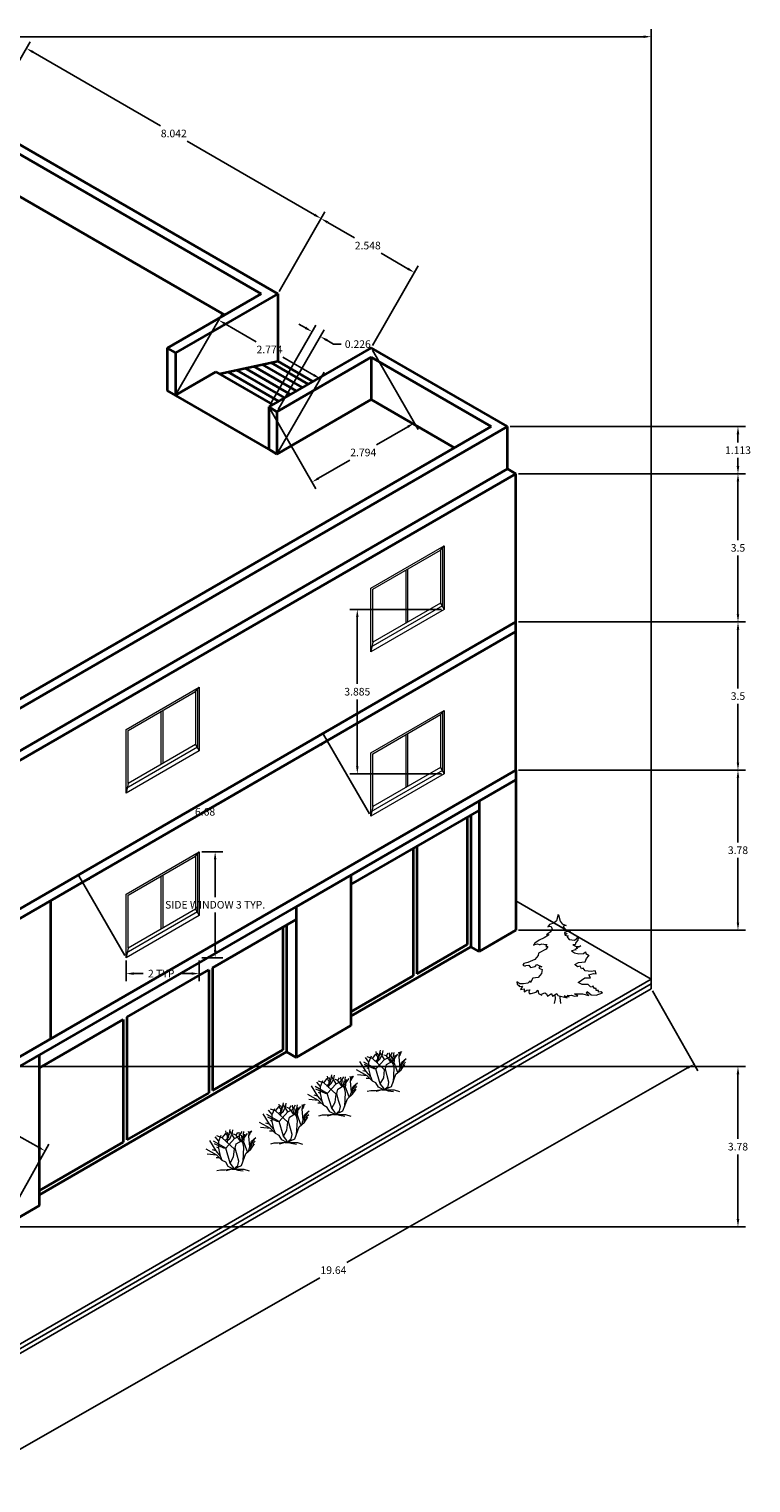
# Model space of a CAD drawing. Units: metres. Extents: x 5057 to 10150, y 1364 to 2760.
# Tile 2 of 2: x 5082 to 5099, y 1364 to 1399. Entities that reach past the tile are written whole.
import ezdxf

# ---------------------------------------------------------------- set-up
doc = ezdxf.new("R2010")
doc.units = ezdxf.units.M
for name, color, linetype, lineweight in [('A-ANNO-DIMS', 2, 'Continuous', 18), ('A-ELEV', 7, 'Continuous', 35), ('A-GLAZ', 4, 'Continuous', 18), ('C-SITE', 3, 'Continuous', 25), ('L-PLNT', 3, 'Continuous', 13)]:
    doc.layers.add(name, color=color, linetype=linetype, lineweight=lineweight)
doc.styles.get("Standard").update_dxf_attribs({"font": 'arial.ttf'})
doc.dimstyles.get("Standard").update_dxf_attribs({"dimtxt": 0.18, "dimasz": 0.18, "dimexe": 0.18, "dimexo": 0.0625, "dimgap": 0.09, "dimtad": 0, "dimtih": 1, "dimtoh": 1, "dimdec": 4, "dimzin": 0, "dimdsep": 46, "dimtxsty": 'Standard', "dimcen": 0.09, "dimadec": 0, "dimazin": 0, "dimtfac": 1, "dimtdec": 4, "dimtofl": 0, "dimtmove": 0, "dimatfit": 3, "dimfxl": 1, "dimtolj": 1, "dimtzin": 0, "dimarcsym": 0})

# ---------------------------------------------------------------- blocks, each defined once
blk = doc.blocks.new('*U4')
for p, q in [((-18.24, 11.04), (-21.755, 16.655)), ((-12.96, 12.48), (-19.68, 16.32)), ((-16.8, 16.32), (-18.72, 18.72)), ((-14.88, 18.24), (-17.76, 19.2)), ((-16.8, 16.32), (-15.36, 19.68)), ((-16.8, 12.48), (-16.8, 16.32)), ((-14.88, 18.24), (-12.96, 20.64)), ((-8.16, 12), (-14.88, 18.24)), ((-13.325, 16.724), (-11.433, 18.289)), ((-12.96, 12.48), (-8.16, 17.76)), ((-12.471, 19.775), (-12.898, 22.044)), ((-11.677, 19.071), (-12.471, 19.775)), ((-11.28, 19.619), (-12.104, 21.184)), ((-12.043, 15.628), (-11.921, 18.836)), ((-11.982, 16.802), (-10.579, 18.054)), ((-11.921, 18.836), (-10.64, 20.401)), ((-11.433, 18.289), (-10.457, 22.749)), ((-10.579, 18.054), (-9.846, 19.697)), ((-8.16, 17.76), (-10.56, 21.6)), ((-9.48, 19.775), (-8.992, 22.592)), ((-7.2, 19.68), (-8.64, 20.16)), ((-8.16, 17.76), (-5.28, 19.2)), ((-7.2, 19.68), (-6.24, 21.12)), ((-4.8, 16.32), (-7.2, 19.68)), ((-7.2, 14.88), (-3.84, 16.8)), ((-5.086, 17.741), (-5.513, 21.34)), ((-5.28, 19.2), (-3.84, 21.6)), ((-3.377, 15.315), (-5.086, 17.819)), ((-2.88, 12.96), (-4.32, 19.68)), ((-3.84, 16.8), (-0.96, 20.64)), ((-3.377, 18.602), (-2.888, 21.575)), ((-2.766, 16.802), (-3.377, 18.602)), ((-2.88, 15.84), (-2.4, 20.16)), ((-0.508, 21.888), (-0.081, 20.558)), ((-0.203, 19.149), (0.102, 21.34)), ((0.346, 13.203), (-0.203, 19.149)), ((-0.142, 19.384), (0.59, 20.401)), ((-0.02, 20.01), (0.896, 21.105)), ((0.041, 20.714), (1.384, 22.044)), ((0.102, 21.34), (0.835, 21.888)), ((0.346, 13.203), (1.323, 16.254)), ((1.323, 16.254), (3.642, 18.289)), ((1.44, 15.36), (2.88, 17.28)), ((2.4, 15.36), (3.36, 16.32)), ((-17.76, 8.64), (-23.663, 11.961)), ((-17.76, 8.64), (-23.128, 9.222)), ((-18.24, 11.04), (-20.16, 11.52)), ((-13.92, 12.48), (-19.2, 14.88)), ((-15.84, 8.16), (-18.24, 11.04)), ((-16.8, 12.48), (-17.76, 12.96)), ((-14.88, 5.76), (-17.76, 8.64)), ((-15.84, 8.16), (-16.8, 12.48)), ((-14.88, 5.76), (-15.84, 8.16)), ((-12.96, 12.48), (-13.92, 12.48)), ((-10.56, 4.32), (-12.96, 12.48)), ((-8.64, 7.68), (-8.16, 12)), ((-7.68, 12.48), (-7.2, 14.88)), ((-6.72, 8.64), (-7.68, 12.48)), ((-5.76, 5.28), (-6.72, 8.64)), ((-4.32, 2.88), (-1.92, 9.6)), ((-3.36, 5.28), (-2.88, 12.96)), ((-0.96, 10.56), (-2.88, 15.84)), ((-1.92, 9.6), (0.96, 12)), ((-0.48, 10.8), (0.346, 13.203)), ((0.96, 12), (1.44, 15.36)), ((0.96, 12), (2.88, 14.88)), ((1.92, 13.44), (2.4, 15.36)), ((-16.32, 7.2), (-18.24, 7.2)), ((-15.84, 0.48), (-17.76, 0)), ((-13.44, 0.48), (-15.84, 0.48)), ((-12.96, 4.8), (-14.88, 5.76)), ((-9.6, 0.96), (-13.44, 0.48)), ((-11.52, 2.4), (-12.96, 4.8)), ((-9.6, 0.96), (-12.96, 0)), ((-8.64, 0.96), (-11.52, 2.4)), ((-10.56, 4.32), (-8.64, 7.68)), ((-8.64, 1.92), (-10.56, 4.32)), ((-9.6, 0.96), (-7.68, 0.96)), ((-8.64, 0.96), (-4.32, 2.88)), ((-8.64, 0.96), (-6.24, 2.88)), ((-8.64, 0.96), (-8.64, 1.92)), ((-8.64, 0.96), (-2.88, 0.96)), ((-7.68, 0.96), (-6.24, 0.48)), ((-6.24, 2.88), (-5.76, 5.28)), ((-6.24, 0.48), (-3.36, 0)), ((-2.88, 0.96), (0, 0))]:
    blk.add_line(p, q)
blk = doc.blocks.new('*U5')
for p, q in [((-9.75, 0), (-8.263, 7.598)), ((-8.263, 7.598), (-8.747, 14.105)), ((-0.771, 9.56), (-0.69, 11.833)), ((0, 0), (-0.771, 9.56))]:
    blk.add_line(p, q)
for points in [[(-3.9, 142.35), (-6.596, 132.037), (-10.801, 128.443), (-17.81, 126.047), (-20.614, 122.452), (-17.81, 123.65), (-15.007, 123.051), (-13.605, 118.858), (-16.876, 114.065), (-21.549, 111.07), (-22.951, 109.872), (-19.212, 110.471), (-19.68, 109.273), (-26.222, 105.079), (-34.633, 101.485), (-41.175, 96.693), (-43.511, 93.098), (-41.175, 94.296), (-36.969, 95.494), (-34.633, 94.296), (-32.764, 94.296), (-29.493, 95.494)], [(-3.759, 141.97), (-1.074, 131.643), (2.437, 127.141), (8.84, 124.493), (6.568, 124.493), (4.09, 123.169), (4.296, 121.846), (7.807, 117.874), (16.069, 116.02), (10.492, 115.226), (5.535, 113.372), (6.981, 112.843), (5.948, 110.989), (10.286, 112.048), (6.775, 109.401), (11.732, 108.077), (9.873, 107.282), (13.797, 102.516), (21.852, 101.192), (25.983, 103.84), (28.048, 106.488), (27.842, 105.164), (27.429, 101.457), (24.124, 97.75), (23.091, 93.513), (19.58, 93.513), (23.505, 91.66), (28.255, 90.866), (31.973, 91.925), (29.081, 89.806), (24.537, 88.747), (26.809, 88.218), (22.472, 86.099), (24.95, 85.57), (17.308, 84.246), (21.852, 80.804), (29.081, 79.215), (36.723, 80.009), (39.821, 82.392), (40.028, 80.009), (45.398, 76.567)], [(-29.25, 95.55), (-25.287, 94.296), (-22.016, 94.296), (-23.885, 91.301), (-20.614, 91.301), (-23.418, 87.108), (-35.567, 80.518), (-36.035, 76.924), (-41.175, 70.334), (-52.389, 65.542), (-58.931, 63.744), (-60.8, 61.348), (-57.062, 59.551), (-56.128, 60.749), (-50.987, 61.348), (-48.184, 57.754), (-40.707, 58.952), (-38.371, 62.546), (-30.427, 58.353), (-33.698, 58.353), (-35.1, 56.556), (-29.493, 54.159), (-30.894, 48.169), (-36.035, 41.579), (-44.446, 40.381), (-48.184, 33.791), (-49.118, 36.188), (-52.857, 32.593), (-59.399, 31.395), (-65.473, 31.395), (-70.146, 34.39), (-69.679, 30.796), (-66.875, 28.999), (-65.941, 27.202), (-61.268, 27.801), (-64.539, 22.409), (-58.464, 23.607), (-58.464, 18.815), (-54.258, 21.211), (-49.586, 21.81), (-50.987, 18.815), (-50.52, 15.82), (-47.249, 15.82), (-39.306, 18.216), (-36.502, 21.211), (-35.567, 15.82), (-30.427, 13.423), (-29.493, 15.221), (-25.287, 17.018), (-22.951, 15.221), (-21.081, 11.626), (-14.539, 15.82), (-13.138, 11.626), (-6.128, 15.82), (-4.726, 12.824), (10.226, 9.23), (5.554, 12.225), (13.497, 10.428), (10.226, 12.824), (16.768, 13.423), (22.376, 11.626), (27.516, 12.225), (21.909, 15.221), (34.993, 15.221), (44.806, 12.824), (41.535, 16.419), (42.469, 19.414), (49.011, 14.023), (56.487, 13.423), (66.768, 17.018), (64.431, 18.815), (60.226, 18.216), (60.226, 20.612), (56.955, 20.612), (56.955, 24.206), (54.151, 24.206), (51.348, 28.4), (50.413, 26.004), (47.609, 26.603), (43.871, 30.197), (38.731, 30.197), (34.525, 30.197), (27.983, 33.791), (38.731, 40.98), (47.609, 40.98), (45.273, 45.773), (52.282, 48.169), (56.955, 47.57), (55.086, 52.362), (48.544, 51.164), (39.198, 52.362), (35.927, 56.556), (33.123, 55.357), (31.254, 59.551), (27.049, 58.353), (22.376, 62.546), (28.451, 65.542), (39.198, 66.74), (41.535, 72.131), (45.273, 76.325)]]:
    blk.add_lwpolyline(points)
blk = doc.blocks.new('WIN-SIDE')
for p, q in [((0, 1.5), (1.732, 2.5)), ((1.646, 2.4), (1.732, 2.5)), ((1.692, 2.453), (1.692, 1.083)), ((1.732, 2.5), (1.732, 1)), ((0.049, 1.478), (1.646, 2.4)), ((1.646, 2.4), (1.646, 1.15)), ((0.826, 1.926), (0.826, 0.676)), ((0.869, 1.951), (0.869, 0.701)), ((0, 0), (0, 1.5)), ((0.049, 0.228), (0.049, 1.478)), ((1.692, 1.083), (0, 0.107)), ((1.646, 1.15), (0.049, 0.228)), ((1.646, 1.15), (1.732, 1)), ((1.732, 1), (0, 0)), ((0.049, 0.228), (0, 0))]:
    blk.add_line(p, q)
blk = doc.blocks.new('*D7')
at = {"layer": 'A-ANNO-DIMS', "color": 0, "lineweight": -2, "transparency": 16777216}
for p, q in [((5085.663, 1379.094), (5086.155, 1379.094)), ((5085.975, 1378.914), (5085.975, 1378.027)), ((5085.975, 1376.774), (5085.975, 1377.66)), ((5085.663, 1376.594), (5086.155, 1376.594))]:
    blk.add_line(p, q, dxfattribs=at)
at = {"layer": 'A-ANNO-DIMS', "color": 0, "transparency": 16777216}
for points in [[(5085.945, 1378.914), (5086.005, 1378.914), (5085.975, 1379.094)], [(5085.945, 1376.774), (5086.005, 1376.774), (5085.975, 1376.594)]]:
    blk.add_solid(points, dxfattribs=at)
at = {"layer": 'Defpoints', "color": 0, "transparency": 16777216}
for p in [(5085.6, 1379.094), (5085.975, 1379.094), (5085.6, 1376.594)]:
    blk.add_point(p, dxfattribs=at)
at = {"layer": 'A-ANNO-DIMS', "color": 0, "transparency": 16777216, "insert": (5085.975, 1377.844), "char_height": 0.18, "attachment_point": 5}
blk.add_mtext('\\A1;SIDE WINDOW 3 TYP.', dxfattribs=at)
blk = doc.blocks.new('*D8')
at = {"layer": 'A-ANNO-DIMS', "color": 0, "lineweight": -2, "transparency": 16777216}
for p, q in [((5083.868, 1376.531), (5083.868, 1376.039)), ((5085.6, 1376.531), (5085.6, 1376.039)), ((5084.048, 1376.219), (5084.275, 1376.219)), ((5085.42, 1376.219), (5085.194, 1376.219))]:
    blk.add_line(p, q, dxfattribs=at)
at = {"layer": 'A-ANNO-DIMS', "color": 0, "transparency": 16777216}
for points in [[(5084.048, 1376.249), (5084.048, 1376.189), (5083.868, 1376.219)], [(5085.42, 1376.249), (5085.42, 1376.189), (5085.6, 1376.219)]]:
    blk.add_solid(points, dxfattribs=at)
at = {"layer": 'Defpoints', "color": 0, "transparency": 16777216}
for p in [(5083.868, 1376.594), (5085.6, 1376.594), (5085.6, 1376.219)]:
    blk.add_point(p, dxfattribs=at)
at = {"layer": 'A-ANNO-DIMS', "color": 0, "transparency": 16777216, "insert": (5084.734, 1376.219), "char_height": 0.18, "attachment_point": 5}
blk.add_mtext('\\A1;2 TYP.', dxfattribs=at)
blk = doc.blocks.new('*D9')
at = {"layer": 'A-ANNO-DIMS', "color": 0, "lineweight": -2, "transparency": 16777216}
for p, q in [((5059.194, 1377.756), (5059.194, 1398.523)), ((5059.374, 1398.343), (5077.345, 1398.343)), ((5096.103, 1398.343), (5078.132, 1398.343)), ((5096.283, 1375.925), (5096.283, 1398.523))]:
    blk.add_line(p, q, dxfattribs=at)
at = {"layer": 'A-ANNO-DIMS', "color": 0, "transparency": 16777216}
for points in [[(5059.374, 1398.373), (5059.374, 1398.313), (5059.194, 1398.343)], [(5096.103, 1398.373), (5096.103, 1398.313), (5096.283, 1398.343)]]:
    blk.add_solid(points, dxfattribs=at)
at = {"layer": 'Defpoints', "color": 0, "transparency": 16777216}
for p in [(5096.283, 1398.343), (5059.194, 1377.694), (5096.283, 1375.863)]:
    blk.add_point(p, dxfattribs=at)
at = {"layer": 'A-ANNO-DIMS', "color": 0, "transparency": 16777216, "insert": (5077.738, 1398.343), "char_height": 0.18, "attachment_point": 5}
blk.add_mtext('\\A1;37.09', dxfattribs=at)
blk = doc.blocks.new('*D12')
at = {"layer": 'A-ANNO-DIMS', "color": 0, "lineweight": -2, "transparency": 16777216}
for p, q in [((5096.314, 1375.808), (5097.388, 1373.926)), ((5097.143, 1373.993), (5089.09, 1369.397)), ((5080.399, 1364.437), (5088.452, 1369.033)), ((5079.257, 1366.074), (5080.332, 1364.191))]:
    blk.add_line(p, q, dxfattribs=at)
at = {"layer": 'A-ANNO-DIMS', "color": 0, "transparency": 16777216}
for points in [[(5097.128, 1374.019), (5097.158, 1373.967), (5097.299, 1374.082)], [(5080.384, 1364.463), (5080.414, 1364.411), (5080.243, 1364.348)]]:
    blk.add_solid(points, dxfattribs=at)
at = {"layer": 'Defpoints', "color": 0, "transparency": 16777216}
for p in [(5096.283, 1375.863), (5079.226, 1366.128), (5080.243, 1364.348)]:
    blk.add_point(p, dxfattribs=at)
at = {"layer": 'A-ANNO-DIMS', "color": 0, "transparency": 16777216, "insert": (5088.771, 1369.215), "char_height": 0.18, "attachment_point": 5}
blk.add_mtext('\\A1;19.64', dxfattribs=at)
blk = doc.blocks.new('*D13')
at = {"layer": 'A-ANNO-DIMS', "color": 0, "lineweight": -2, "transparency": 16777216}
for p, q in [((5093.145, 1381.022), (5098.513, 1381.022)), ((5098.333, 1380.842), (5098.333, 1379.314)), ((5098.333, 1377.421), (5098.333, 1378.95)), ((5093.145, 1377.241), (5098.513, 1377.241))]:
    blk.add_line(p, q, dxfattribs=at)
at = {"layer": 'A-ANNO-DIMS', "color": 0, "transparency": 16777216}
for points in [[(5098.303, 1380.842), (5098.363, 1380.842), (5098.333, 1381.022)], [(5098.303, 1377.421), (5098.363, 1377.421), (5098.333, 1377.241)]]:
    blk.add_solid(points, dxfattribs=at)
at = {"layer": 'Defpoints', "color": 0, "transparency": 16777216}
for p in [(5093.083, 1381.022), (5098.333, 1381.022), (5093.083, 1377.241)]:
    blk.add_point(p, dxfattribs=at)
at = {"layer": 'A-ANNO-DIMS', "color": 0, "transparency": 16777216, "insert": (5098.333, 1379.132), "char_height": 0.18, "attachment_point": 5}
blk.add_mtext('\\A1;3.78', dxfattribs=at)
blk = doc.blocks.new('*D14')
at = {"layer": 'A-ANNO-DIMS', "color": 0, "lineweight": -2, "transparency": 16777216}
for p, q in [((5093.145, 1384.522), (5098.513, 1384.522)), ((5098.333, 1384.342), (5098.333, 1382.954)), ((5098.333, 1381.202), (5098.333, 1382.59)), ((5093.145, 1381.022), (5098.513, 1381.022))]:
    blk.add_line(p, q, dxfattribs=at)
at = {"layer": 'A-ANNO-DIMS', "color": 0, "transparency": 16777216}
for points in [[(5098.303, 1384.342), (5098.363, 1384.342), (5098.333, 1384.522)], [(5098.303, 1381.202), (5098.363, 1381.202), (5098.333, 1381.022)]]:
    blk.add_solid(points, dxfattribs=at)
at = {"layer": 'Defpoints', "color": 0, "transparency": 16777216}
for p in [(5093.083, 1384.522), (5098.333, 1384.522), (5093.083, 1381.022)]:
    blk.add_point(p, dxfattribs=at)
at = {"layer": 'A-ANNO-DIMS', "color": 0, "transparency": 16777216, "insert": (5098.333, 1382.772), "char_height": 0.18, "attachment_point": 5}
blk.add_mtext('\\A1;3.5', dxfattribs=at)
blk = doc.blocks.new('*D15')
at = {"layer": 'A-ANNO-DIMS', "color": 0, "lineweight": -2, "transparency": 16777216}
for p, q in [((5093.145, 1388.022), (5098.513, 1388.022)), ((5098.333, 1387.842), (5098.333, 1386.454)), ((5098.333, 1384.702), (5098.333, 1386.09)), ((5093.145, 1384.522), (5098.513, 1384.522))]:
    blk.add_line(p, q, dxfattribs=at)
at = {"layer": 'A-ANNO-DIMS', "color": 0, "transparency": 16777216}
for points in [[(5098.303, 1387.842), (5098.363, 1387.842), (5098.333, 1388.022)], [(5098.303, 1384.702), (5098.363, 1384.702), (5098.333, 1384.522)]]:
    blk.add_solid(points, dxfattribs=at)
at = {"layer": 'Defpoints', "color": 0, "transparency": 16777216}
for p in [(5093.083, 1388.022), (5098.333, 1388.022), (5093.083, 1384.522)]:
    blk.add_point(p, dxfattribs=at)
at = {"layer": 'A-ANNO-DIMS', "color": 0, "transparency": 16777216, "insert": (5098.333, 1386.272), "char_height": 0.18, "attachment_point": 5}
blk.add_mtext('\\A1;3.5', dxfattribs=at)
blk = doc.blocks.new('*D16')
at = {"layer": 'A-ANNO-DIMS', "color": 0, "lineweight": -2, "transparency": 16777216}
for p, q in [((5092.95, 1389.135), (5098.513, 1389.135)), ((5098.333, 1388.955), (5098.333, 1388.761)), ((5098.333, 1388.202), (5098.333, 1388.397)), ((5093.145, 1388.022), (5098.513, 1388.022))]:
    blk.add_line(p, q, dxfattribs=at)
at = {"layer": 'A-ANNO-DIMS', "color": 0, "transparency": 16777216}
for points in [[(5098.303, 1388.955), (5098.363, 1388.955), (5098.333, 1389.135)], [(5098.303, 1388.202), (5098.363, 1388.202), (5098.333, 1388.022)]]:
    blk.add_solid(points, dxfattribs=at)
at = {"layer": 'Defpoints', "color": 0, "transparency": 16777216}
for p in [(5092.887, 1389.135), (5098.333, 1389.135), (5093.083, 1388.022)]:
    blk.add_point(p, dxfattribs=at)
at = {"layer": 'A-ANNO-DIMS', "color": 0, "transparency": 16777216, "insert": (5098.333, 1388.579), "char_height": 0.18, "attachment_point": 5}
blk.add_mtext('\\A1;1.113', dxfattribs=at)
blk = doc.blocks.new('*D17')
at = {"layer": 'A-ANNO-DIMS', "color": 0, "lineweight": -2, "transparency": 16777216}
for p, q in [((5080.521, 1396.347), (5081.604, 1398.224)), ((5081.67, 1397.979), (5084.681, 1396.24)), ((5088.323, 1394.138), (5085.312, 1395.876)), ((5087.485, 1392.327), (5088.569, 1394.204))]:
    blk.add_line(p, q, dxfattribs=at)
at = {"layer": 'A-ANNO-DIMS', "color": 0, "transparency": 16777216}
for points in [[(5081.685, 1398.005), (5081.655, 1397.953), (5081.514, 1398.069)], [(5088.338, 1394.164), (5088.308, 1394.112), (5088.479, 1394.048)]]:
    blk.add_solid(points, dxfattribs=at)
at = {"layer": 'Defpoints', "color": 0, "transparency": 16777216}
for p in [(5080.489, 1396.293), (5088.479, 1394.048), (5087.454, 1392.272)]:
    blk.add_point(p, dxfattribs=at)
at = {"layer": 'A-ANNO-DIMS', "color": 0, "transparency": 16777216, "insert": (5084.997, 1396.058), "char_height": 0.18, "attachment_point": 5}
blk.add_mtext('\\A1;8.042', dxfattribs=at)
blk = doc.blocks.new('*D18')
at = {"layer": 'A-ANNO-DIMS', "color": 0, "lineweight": -2, "transparency": 16777216}
for p, q in [((5087.485, 1392.327), (5088.569, 1394.204)), ((5088.635, 1393.958), (5089.267, 1393.593)), ((5090.529, 1392.864), (5089.897, 1393.229)), ((5089.692, 1391.053), (5090.775, 1392.93))]:
    blk.add_line(p, q, dxfattribs=at)
at = {"layer": 'A-ANNO-DIMS', "color": 0, "transparency": 16777216}
for points in [[(5088.65, 1393.984), (5088.62, 1393.932), (5088.479, 1394.048)], [(5090.544, 1392.89), (5090.514, 1392.838), (5090.685, 1392.774)]]:
    blk.add_solid(points, dxfattribs=at)
at = {"layer": 'Defpoints', "color": 0, "transparency": 16777216}
for p in [(5090.685, 1392.774), (5087.454, 1392.272), (5089.66, 1390.998)]:
    blk.add_point(p, dxfattribs=at)
at = {"layer": 'A-ANNO-DIMS', "color": 0, "transparency": 16777216, "insert": (5089.582, 1393.411), "char_height": 0.18, "attachment_point": 5}
blk.add_mtext('\\A1;2.548', dxfattribs=at)
blk = doc.blocks.new('*D19')
at = {"layer": 'A-ANNO-DIMS', "color": 0, "lineweight": -2, "transparency": 16777216}
for p, q in [((5089.692, 1390.944), (5090.775, 1389.067)), ((5087.272, 1389.547), (5088.356, 1387.67)), ((5090.529, 1389.133), (5089.79, 1388.706)), ((5088.421, 1387.916), (5089.16, 1388.343))]:
    blk.add_line(p, q, dxfattribs=at)
at = {"layer": 'A-ANNO-DIMS', "color": 0, "transparency": 16777216}
for points in [[(5090.514, 1389.159), (5090.544, 1389.107), (5090.685, 1389.223)], [(5088.406, 1387.942), (5088.436, 1387.89), (5088.266, 1387.826)]]:
    blk.add_solid(points, dxfattribs=at)
at = {"layer": 'Defpoints', "color": 0, "transparency": 16777216}
for p in [(5089.66, 1390.998), (5087.241, 1389.601), (5088.266, 1387.826)]:
    blk.add_point(p, dxfattribs=at)
at = {"layer": 'A-ANNO-DIMS', "color": 0, "transparency": 16777216, "insert": (5089.475, 1388.525), "char_height": 0.18, "attachment_point": 5}
blk.add_mtext('\\A1;2.794', dxfattribs=at)
blk = doc.blocks.new('*D20')
at = {"layer": 'A-ANNO-DIMS', "color": 0, "lineweight": -2, "transparency": 16777216}
for p, q in [((5087.272, 1389.655), (5088.356, 1391.533)), ((5088.11, 1391.467), (5087.954, 1391.557)), ((5087.468, 1389.542), (5088.551, 1391.42)), ((5088.617, 1391.174), (5088.773, 1391.084)), ((5088.773, 1391.084), (5088.953, 1391.084))]:
    blk.add_line(p, q, dxfattribs=at)
at = {"layer": 'A-ANNO-DIMS', "color": 0, "transparency": 16777216}
for points in [[(5088.125, 1391.493), (5088.095, 1391.441), (5088.266, 1391.377)], [(5088.632, 1391.2), (5088.602, 1391.148), (5088.461, 1391.264)]]:
    blk.add_solid(points, dxfattribs=at)
at = {"layer": 'Defpoints', "color": 0, "transparency": 16777216}
for p in [(5088.461, 1391.264), (5087.241, 1389.601), (5087.436, 1389.488)]:
    blk.add_point(p, dxfattribs=at)
at = {"layer": 'A-ANNO-DIMS', "color": 0, "transparency": 16777216, "insert": (5089.347, 1391.084), "char_height": 0.18, "attachment_point": 5}
blk.add_mtext('\\A1;0.226', dxfattribs=at)
blk = doc.blocks.new('*D21')
at = {"layer": 'A-ANNO-DIMS', "color": 0, "lineweight": -2, "transparency": 16777216}
for p, q in [((5085.065, 1389.929), (5086.149, 1391.807)), ((5086.215, 1391.561), (5086.948, 1391.138)), ((5088.305, 1390.354), (5087.572, 1390.777)), ((5087.468, 1388.542), (5088.551, 1390.42))]:
    blk.add_line(p, q, dxfattribs=at)
at = {"layer": 'A-ANNO-DIMS', "color": 0, "transparency": 16777216}
for points in [[(5086.23, 1391.587), (5086.2, 1391.535), (5086.059, 1391.651)], [(5088.32, 1390.38), (5088.29, 1390.328), (5088.461, 1390.264)]]:
    blk.add_solid(points, dxfattribs=at)
at = {"layer": 'Defpoints', "color": 0, "transparency": 16777216}
for p in [(5088.461, 1390.264), (5085.034, 1389.875), (5087.436, 1388.488)]:
    blk.add_point(p, dxfattribs=at)
at = {"layer": 'A-ANNO-DIMS', "color": 0, "transparency": 16777216, "insert": (5087.26, 1390.957), "char_height": 0.18, "attachment_point": 5}
blk.add_mtext('\\A1;2.774', dxfattribs=at)
blk = doc.blocks.new('*D22')
at = {"layer": 'A-ANNO-DIMS', "color": 0, "lineweight": -2, "transparency": 16777216}
for p, q in [((5089.622, 1379.988), (5088.538, 1381.865)), ((5088.472, 1381.619), (5086.051, 1380.221)), ((5082.999, 1378.459), (5085.421, 1379.857)), ((5083.837, 1376.648), (5082.753, 1378.525))]:
    blk.add_line(p, q, dxfattribs=at)
at = {"layer": 'A-ANNO-DIMS', "color": 0, "transparency": 16777216}
for points in [[(5088.457, 1381.645), (5088.487, 1381.593), (5088.628, 1381.709)], [(5082.984, 1378.485), (5083.014, 1378.433), (5082.843, 1378.369)]]:
    blk.add_solid(points, dxfattribs=at)
at = {"layer": 'Defpoints', "color": 0, "transparency": 16777216}
for p in [(5088.628, 1381.709), (5089.653, 1379.934), (5083.868, 1376.594)]:
    blk.add_point(p, dxfattribs=at)
at = {"layer": 'A-ANNO-DIMS', "color": 0, "transparency": 16777216, "insert": (5085.736, 1380.039), "char_height": 0.18, "attachment_point": 5}
blk.add_mtext('\\A1;6.68', dxfattribs=at)
blk = doc.blocks.new('*D23')
at = {"layer": 'A-ANNO-DIMS', "color": 0, "lineweight": -2, "transparency": 16777216}
for p, q in [((5091.323, 1384.819), (5089.155, 1384.819)), ((5089.335, 1384.639), (5089.335, 1383.058)), ((5089.335, 1381.114), (5089.335, 1382.694)), ((5091.323, 1380.934), (5089.155, 1380.934))]:
    blk.add_line(p, q, dxfattribs=at)
at = {"layer": 'A-ANNO-DIMS', "color": 0, "transparency": 16777216}
for points in [[(5089.305, 1384.639), (5089.365, 1384.639), (5089.335, 1384.819)], [(5089.305, 1381.114), (5089.365, 1381.114), (5089.335, 1380.934)]]:
    blk.add_solid(points, dxfattribs=at)
at = {"layer": 'Defpoints', "color": 0, "transparency": 16777216}
for p in [(5089.335, 1384.819), (5091.385, 1384.819), (5091.385, 1380.934)]:
    blk.add_point(p, dxfattribs=at)
at = {"layer": 'A-ANNO-DIMS', "color": 0, "transparency": 16777216, "insert": (5089.335, 1382.876), "char_height": 0.18, "attachment_point": 5}
blk.add_mtext('\\A1;3.885', dxfattribs=at)
blk = doc.blocks.new('*D27')
at = {"layer": 'A-ANNO-DIMS', "color": 0, "lineweight": -2, "transparency": 16777216}
for p, q in [((5075.911, 1373.114), (5076.963, 1375.009)), ((5077.033, 1374.765), (5079.087, 1373.625)), ((5081.796, 1372.121), (5079.742, 1373.261)), ((5080.989, 1370.296), (5082.041, 1372.191))]:
    blk.add_line(p, q, dxfattribs=at)
at = {"layer": 'A-ANNO-DIMS', "color": 0, "transparency": 16777216}
for points in [[(5077.048, 1374.791), (5077.019, 1374.738), (5076.876, 1374.852)], [(5081.811, 1372.147), (5081.781, 1372.095), (5081.953, 1372.033)]]:
    blk.add_solid(points, dxfattribs=at)
at = {"layer": 'Defpoints', "color": 0, "transparency": 16777216}
for p in [(5075.881, 1373.06), (5081.953, 1372.033), (5080.958, 1370.241)]:
    blk.add_point(p, dxfattribs=at)
at = {"layer": 'A-ANNO-DIMS', "color": 0, "transparency": 16777216, "insert": (5079.415, 1373.443), "char_height": 0.18, "attachment_point": 5}
blk.add_mtext('\\A1;5.807', dxfattribs=at)
blk = doc.blocks.new('*D28')
at = {"layer": 'A-ANNO-DIMS', "color": 0, "lineweight": -2, "transparency": 16777216}
for p, q in [((5081.021, 1374.022), (5098.513, 1374.022)), ((5098.333, 1373.842), (5098.333, 1372.314)), ((5098.333, 1370.421), (5098.333, 1371.95)), ((5081.021, 1370.241), (5098.513, 1370.241))]:
    blk.add_line(p, q, dxfattribs=at)
at = {"layer": 'A-ANNO-DIMS', "color": 0, "transparency": 16777216}
for points in [[(5098.303, 1373.842), (5098.363, 1373.842), (5098.333, 1374.022)], [(5098.303, 1370.421), (5098.363, 1370.421), (5098.333, 1370.241)]]:
    blk.add_solid(points, dxfattribs=at)
at = {"layer": 'Defpoints', "color": 0, "transparency": 16777216}
for p in [(5080.958, 1374.022), (5098.333, 1374.022), (5080.958, 1370.241)]:
    blk.add_point(p, dxfattribs=at)
at = {"layer": 'A-ANNO-DIMS', "color": 0, "transparency": 16777216, "insert": (5098.333, 1372.132), "char_height": 0.18, "attachment_point": 5}
blk.add_mtext('\\A1;3.78', dxfattribs=at)

msp = doc.modelspace()

# ---------------------------------------------------------------- linework, layer by layer
at = {"layer": 'A-ELEV'}
for p, q in [((5087.4536, 1392.2724), (5080.4894, 1396.2932)), ((5087.0622, 1392.2724), (5080.4894, 1396.0672)), ((5080.4894, 1395.0672), (5086.1962, 1391.7724)), ((5087.0622, 1392.2724), (5084.8382, 1390.9884)), ((5087.4536, 1392.2724), (5085.0339, 1390.8754)), ((5087.4536, 1392.2724), (5087.4536, 1390.6823)), ((5087.4536, 1392.2724), (5087.4536, 1390.6823)), ((5084.8382, 1390.9884), (5085.0339, 1390.8754)), ((5084.8382, 1390.9884), (5084.8382, 1389.9884)), ((5085.0339, 1390.8754), (5085.0339, 1389.8754)), ((5089.6603, 1390.9984), (5087.2405, 1389.6014)), ((5092.8871, 1389.1354), (5089.6603, 1390.9984)), ((5086.0724, 1390.3834), (5087.4536, 1390.6823)), ((5086.4783, 1390.4712), (5087.6127, 1389.8162)), ((5086.6812, 1390.5151), (5087.7522, 1389.8968)), ((5086.8842, 1390.5591), (5087.8917, 1389.9773)), ((5087.0871, 1390.603), (5088.0313, 1390.0579)), ((5087.2901, 1390.6469), (5088.1708, 1390.1384)), ((5089.6603, 1390.7724), (5087.4363, 1389.4884)), ((5087.4536, 1390.6823), (5088.2832, 1390.2033)), ((5092.4956, 1389.1354), (5089.6603, 1390.7724)), ((5089.6603, 1390.7724), (5089.6603, 1389.7724)), ((5085.0339, 1389.8754), (5085.9931, 1390.4291)), ((5085.9931, 1390.4291), (5087.3337, 1389.6551)), ((5086.2753, 1390.4273), (5087.4732, 1389.7357)), ((5087.2405, 1388.6014), (5084.8382, 1389.9884)), ((5089.6603, 1389.7724), (5087.4363, 1388.4884)), ((5089.6603, 1389.7724), (5091.6296, 1388.6354)), ((5087.2405, 1389.6014), (5087.4363, 1389.4884)), ((5087.2405, 1389.6014), (5087.2405, 1388.6014)), ((5087.4363, 1389.4884), (5087.4363, 1388.4884)), ((5081.3272, 1382.4613), (5092.8871, 1389.1354)), ((5081.3272, 1382.6873), (5092.4956, 1389.1354)), ((5092.8871, 1388.1354), (5092.8871, 1389.1354)), ((5087.4363, 1388.4884), (5087.2405, 1388.6014)), ((5081.1315, 1381.3483), (5092.8871, 1388.1354)), ((5093.0828, 1388.0224), (5092.8871, 1388.1354)), ((5081.3272, 1381.2353), (5093.0828, 1388.0224)), ((5093.0828, 1381.0224), (5093.0828, 1388.0224)), ((5080.8583, 1377.4646), (5093.0828, 1384.5224)), ((5080.8583, 1377.2386), (5093.0828, 1384.2964)), ((5080.9585, 1374.0224), (5093.0828, 1381.0224)), ((5093.0828, 1381.0224), (5093.0828, 1377.241)), ((5087.8867, 1377.7964), (5093.0828, 1380.7964)), ((5092.2168, 1380.2964), (5092.2168, 1376.741)), ((5089.1857, 1378.3204), (5092.2168, 1380.0704)), ((5091.9345, 1379.9074), (5091.9345, 1376.904)), ((5092.0211, 1379.9574), (5092.0211, 1376.854)), ((5090.6579, 1379.1704), (5090.6579, 1376.167)), ((5090.7445, 1379.2204), (5090.7445, 1376.217)), ((5089.1857, 1378.5464), (5089.1857, 1374.991)), ((5080.9585, 1373.7964), (5087.8867, 1377.7964)), ((5082.081, 1377.9445), (5082.081, 1374.6705)), ((5087.8867, 1377.7964), (5087.8867, 1374.241)), ((5085.9092, 1376.3547), (5087.8867, 1377.4964)), ((5087.5775, 1377.3179), (5087.5775, 1374.4195)), ((5087.6641, 1377.3679), (5087.6641, 1374.3695)), ((5092.2168, 1376.741), (5093.0828, 1377.241)), ((5092.0211, 1376.854), (5089.1857, 1375.217)), ((5091.9345, 1376.904), (5090.7445, 1376.217)), ((5092.2168, 1376.741), (5092.0211, 1376.854)), ((5083.8885, 1375.1881), (5085.8226, 1376.3047)), ((5085.8226, 1376.3047), (5085.8226, 1373.4063)), ((5085.9092, 1376.3547), (5085.9092, 1373.4563)), ((5090.6579, 1376.167), (5089.1857, 1375.317)), ((5081.8245, 1373.9964), (5083.8019, 1375.1381)), ((5083.8019, 1375.1381), (5083.8019, 1372.2396)), ((5083.8885, 1375.1881), (5083.8885, 1372.2896)), ((5087.8867, 1374.241), (5089.1857, 1374.991)), ((5087.6641, 1374.3695), (5081.8245, 1370.998)), ((5087.5775, 1374.4195), (5085.9092, 1373.4563)), ((5087.8867, 1374.241), (5087.6641, 1374.3695)), ((5081.8245, 1370.741), (5081.8245, 1374.2964)), ((5085.8226, 1373.4063), (5083.8885, 1372.2896)), ((5083.8019, 1372.2396), (5081.8245, 1371.098)), ((5080.9585, 1370.241), (5081.8245, 1370.741))]:
    msp.add_line(p, q, dxfattribs=at)
at = {"layer": 'C-SITE'}
for p, q in [((5093.0828, 1377.9363), (5096.283, 1376.0886)), ((5079.2264, 1366.241), (5096.283, 1376.0886)), ((5096.283, 1376.0886), (5096.283, 1375.8626)), ((5079.2264, 1366.128), (5096.283, 1375.9756)), ((5079.2264, 1366.015), (5096.283, 1375.8626))]:
    msp.add_line(p, q, dxfattribs=at)

# ---------------------------------------------------------------- block references
at = {"layer": 'A-GLAZ'}
for p in [(5089.6529, 1383.8192), (5083.868, 1380.4793), (5089.6529, 1379.9339), (5083.868, 1376.594)]:
    msp.add_blockref('WIN-SIDE', p, dxfattribs=at)
at = {"layer": 'L-PLNT'}
for name, p, xscale, yscale, zscale in [('*U5', (5094.1428, 1375.513), 0.0147697621143335, 0.0147697621143335, 0.0147697621143335), ('*U4', (5090.3311, 1373.4306), 0.0429228382341487, 0.0429228382341487, 0.0429228382341487), ('*U4', (5089.1822, 1372.8532), 0.0429228382341487, 0.0429228382341487, 0.0429228382341487), ('*U4', (5088.0418, 1372.1919), 0.0429228382341487, 0.0429228382341487, 0.0429228382341487), ('*U4', (5086.78, 1371.5601), 0.0429228382341487, 0.0429228382341487, 0.0429228382341487)]:
    msp.add_blockref(name, p, dxfattribs=dict(at, xscale=xscale, yscale=yscale, zscale=zscale))

# ---------------------------------------------------------------- dimensions: what is measured, and where the dimension line sits
at = {"layer": 'A-ANNO-DIMS'}
dim = msp.add_linear_dim(base=(5096.283, 1398.3432), p1=(5059.194, 1377.6937), p2=(5096.283, 1375.8626), dimstyle='Standard', override={"dimdec": 2, "dimlfac": 1, "dimrnd": 0, "dimzin": 0, "dimdsep": 46, "dimlunit": 2}, dxfattribs=at)
dim.commit()
dim.dimension.update_dxf_attribs({"geometry": '*D9', "text_midpoint": (5077.7385, 1398.3432)})
for base, p1, p2, angle, override, picture, middle in [((5088.4786, 1394.0478), (5080.4894, 1396.2932), (5087.4536, 1392.2724), 330, {"dimdec": 3, "dimlfac": 1, "dimrnd": 0, "dimzin": 0, "dimdsep": 46, "dimlunit": 2}, '*D17', (5084.9965, 1396.0582)), ((5090.6853, 1392.7738), (5087.4536, 1392.2724), (5089.6603, 1390.9984), 330, {"dimdec": 3, "dimlfac": 1, "dimrnd": 0, "dimzin": 0, "dimdsep": 46, "dimlunit": 2}, '*D18', (5089.582, 1393.4108)), ((5088.4613, 1390.2637), (5085.0339, 1389.8754), (5087.4363, 1388.4884), 330, {"dimdec": 3, "dimlfac": 1, "dimrnd": 0, "dimzin": 0, "dimdsep": 46, "dimlunit": 2}, '*D21', (5087.2601, 1390.9572)), ((5088.4613, 1391.2637), (5087.2405, 1389.6014), (5087.4363, 1389.4884), 330, {"dimdec": 3, "dimlfac": 1, "dimrnd": 0, "dimzin": 0, "dimdsep": 46, "dimlunit": 2}, '*D20', (5089.3467, 1391.0837)), ((5088.2655, 1387.826), (5089.6603, 1390.9984), (5087.2405, 1389.6014), 210, {"dimdec": 3, "dimlfac": 1, "dimrnd": 0, "dimzin": 0, "dimdsep": 46, "dimlunit": 2}, '*D19', (5089.4754, 1388.5245)), ((5098.333, 1389.1354), (5093.0828, 1388.0224), (5092.8871, 1389.1354), 90, {"dimdec": 3, "dimlfac": 1, "dimrnd": 0, "dimzin": 0, "dimdsep": 46, "dimlunit": 2}, '*D16', (5098.333, 1388.5789)), ((5098.333, 1388.0224), (5093.0828, 1384.5224), (5093.0828, 1388.0224), 90, {"dimdec": 1, "dimlfac": 1, "dimrnd": 0, "dimzin": 0, "dimdsep": 46, "dimlunit": 2}, '*D15', (5098.333, 1386.2724)), ((5089.3353, 1384.8189), (5091.3853, 1380.9335), (5091.3853, 1384.8189), 90, {"dimdec": 3, "dimlfac": 1, "dimrnd": 0, "dimzin": 0, "dimdsep": 46, "dimlunit": 2}, '*D23', (5089.3353, 1382.8762)), ((5098.333, 1384.5224), (5093.0828, 1381.0224), (5093.0828, 1384.5224), 90, {"dimdec": 1, "dimlfac": 1, "dimrnd": 0, "dimzin": 0, "dimdsep": 46, "dimlunit": 2}, '*D14', (5098.333, 1382.7724)), ((5088.6282, 1381.7089), (5083.8684, 1376.5937), (5089.6532, 1379.9335), 30, {"dimdec": 2, "dimlfac": 1, "dimrnd": 0, "dimzin": 0, "dimdsep": 46, "dimlunit": 2}, '*D22', (5085.7358, 1380.039)), ((5098.333, 1381.0224), (5093.0828, 1377.241), (5093.0828, 1381.0224), 90, {"dimdec": 2, "dimlfac": 1, "dimrnd": 0, "dimzin": 0, "dimdsep": 46, "dimlunit": 2}, '*D13', (5098.333, 1379.1317)), ((5080.2425, 1364.3476), (5096.283, 1375.8626), (5079.2264, 1366.128), 209.71449, {"dimdec": 2, "dimlfac": 1, "dimrnd": 0, "dimzin": 0, "dimdsep": 46, "dimlunit": 2}, '*D12', (5088.7708, 1369.2149)), ((5081.9534, 1372.0334), (5075.8809, 1373.0595), (5080.9585, 1370.241), 330.96555, {"dimdec": 3, "dimlfac": 1, "dimrnd": 0, "dimzin": 0, "dimdsep": 46, "dimlunit": 2}, '*D27', (5079.4146, 1373.4426)), ((5098.333, 1374.0224), (5080.9585, 1370.241), (5080.9585, 1374.0224), 90, {"dimdec": 2, "dimlfac": 1, "dimrnd": 0, "dimzin": 0, "dimdsep": 46, "dimlunit": 2}, '*D28', (5098.333, 1372.1317))]:
    dim = msp.add_linear_dim(base=base, p1=p1, p2=p2, angle=angle, dimstyle='Standard', override=override, dxfattribs=at)
    dim.commit()
    dim.dimension.update_dxf_attribs({"geometry": picture, "text_midpoint": middle})
dim = msp.add_linear_dim(base=(5085.9754321403, 1379.0936564171), p1=(5085.6004321403, 1376.5936564171), p2=(5085.6004321403, 1379.0936564171), angle=90, text='SIDE WINDOW <> TYP.', dimstyle='Standard', override={"dimdec": 0, "dimlfac": 1, "dimrnd": 0, "dimzin": 0, "dimdsep": 46, "dimlunit": 2}, dxfattribs=at)
dim.commit()
dim.dimension.update_dxf_attribs({"geometry": '*D7', "text_midpoint": (5085.9754321403, 1377.8436564171)})
dim = msp.add_linear_dim(base=(5085.6004, 1376.2187), p1=(5083.8684, 1376.5937), p2=(5085.6004, 1376.5937), text='<> TYP.', dimstyle='Standard', override={"dimdec": 0, "dimlfac": 1, "dimrnd": 0, "dimzin": 0, "dimdsep": 46, "dimlunit": 2}, dxfattribs=at)
dim.commit()
dim.dimension.update_dxf_attribs({"geometry": '*D8', "text_midpoint": (5084.7344, 1376.2187)})

doc.saveas('drawing.dxf')
